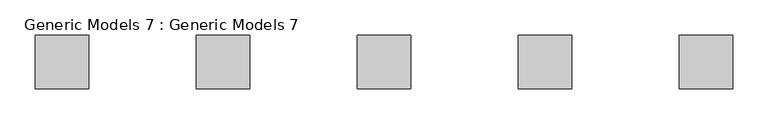
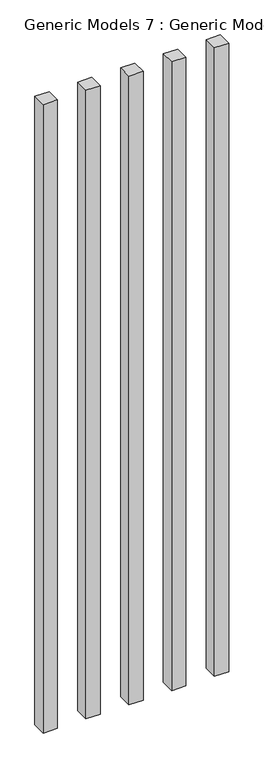
"""IFC4 building model written with IfcOpenShell, lengths in millimetres: proxy geometry, Generic Models 7 : Generic Models 7."""

from ifc_helpers import new_model, si_unit, frame, origin, place, context, project, spatial, polyline, outline, extrude, source, transform, mapped, element, save


def generic_models_7_generic_models_7_f5532255(model_context):
    return source(origin(), model_context, "Body", "SweptSolid", [
        extrude(outline(polyline([(3400.6376365, -13144.1643494), (3400.6376365, -13067.9643494), (3476.8376365, -13067.9643494), (3476.8376365, -13144.1643494), (3400.6376365, -13144.1643494)])), frame((0.0, 0.0, 4289.7327509), z_axis=(0.0, 0.0, 1.0), x_axis=(1.0, 0.0, 0.0)), (0.0, 0.0, 1.0), 3549.6608336),
        extrude(outline(polyline([(3629.2376365, -13144.1643494), (3629.2376365, -13067.9643494), (3705.4376365, -13067.9643494), (3705.4376365, -13144.1643494), (3629.2376365, -13144.1643494)])), frame((0.0, 0.0, 4289.7327509), z_axis=(0.0, 0.0, 1.0), x_axis=(1.0, 0.0, 0.0)), (0.0, 0.0, 1.0), 3549.6608336),
        extrude(outline(polyline([(3857.8376365, -13144.1643494), (3857.8376365, -13067.9643494), (3934.0376365, -13067.9643494), (3934.0376365, -13144.1643494), (3857.8376365, -13144.1643494)])), frame((0.0, 0.0, 4289.7327509), z_axis=(0.0, 0.0, 1.0), x_axis=(1.0, 0.0, 0.0)), (0.0, 0.0, 1.0), 3549.6608336),
        extrude(outline(polyline([(4086.4376365, -13144.1643494), (4086.4376365, -13067.9643494), (4162.6376365, -13067.9643494), (4162.6376365, -13144.1643494), (4086.4376365, -13144.1643494)])), frame((0.0, 0.0, 4289.7327509), z_axis=(0.0, 0.0, 1.0), x_axis=(1.0, 0.0, 0.0)), (0.0, 0.0, 1.0), 3549.6608336),
        extrude(outline(polyline([(4315.0376365, -13144.1643494), (4315.0376365, -13067.9643494), (4391.2376365, -13067.9643494), (4391.2376365, -13144.1643494), (4315.0376365, -13144.1643494)])), frame((0.0, 0.0, 4289.7327509), z_axis=(0.0, 0.0, 1.0), x_axis=(1.0, 0.0, 0.0)), (0.0, 0.0, 1.0), 3549.6608336),
    ])


if __name__ == "__main__":
    model = new_model("IFC4")
    model_context = context("Model", 3, world=origin())
    ifc_project = project(units=[si_unit("LENGTHUNIT", "METRE", prefix="MILLI")], contexts=[model_context])
    site = spatial("IfcSite", under=ifc_project)
    building = spatial("IfcBuilding", under=site)
    placement = place(None, origin())
    generic_models_7_generic_models_7_shape = generic_models_7_generic_models_7_f5532255(model_context)
    element("IfcBuildingElementProxy", 1, Name="Generic Models 7 : Generic Models 7", ObjectType="Generic Models 7 : Generic Models 7", at=placement, inside=building, context=model_context, shape_type="MappedRepresentation", body=[
        mapped(generic_models_7_generic_models_7_shape, transform((0.0, 0.0, 0.0), x_axis=(1.0, 0.0, 0.0), y_axis=(0.0, 1.0, 0.0), z_axis=(0.0, 0.0, 1.0))),
    ])
    save(model, "model.ifc")
